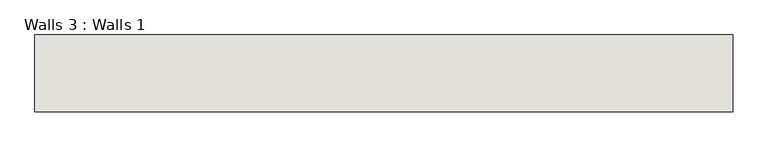
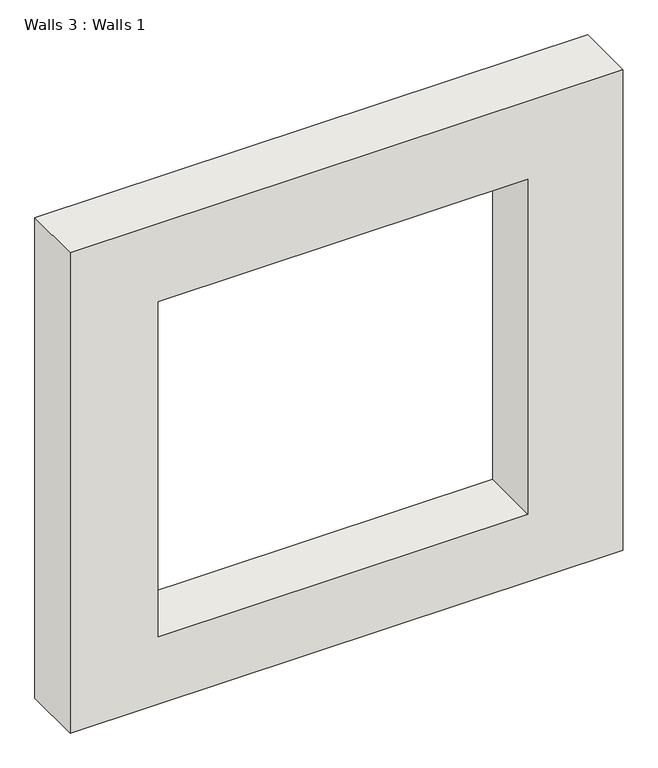
"""IFC4 building model written with IfcOpenShell, lengths in millimetres: wall geometry, Walls 3 : Walls 1."""

from ifc_helpers import new_model, si_unit, frame, origin, place, context, project, spatial, polyline, outline, extrude, source, transform, mapped, element, save


def walls_3_walls_1_8b7cdd2a(model_context):
    return source(origin(), model_context, "Body", "SweptSolid", [
        extrude(outline(polyline([(10639.5789316, -6069.6817469), (10639.5789316, -8558.8817469), (8353.5789316, -8558.8817469), (8353.5789316, -6069.6817469), (10639.5789316, -6069.6817469)]), holes=[polyline([(10268.0681256, -6498.1357575), (8674.2181256, -6498.1357575), (8674.2181256, -8161.8357575), (10268.0681256, -8161.8357575), (10268.0681256, -6498.1357575)])]), frame((0.0, 1408.0209854, 0.0), z_axis=(0.0, 1.0, 0.0), x_axis=(0.0, 0.0, 1.0)), (0.0, 0.0, 1.0), 274.2274628),
    ])


if __name__ == "__main__":
    model = new_model("IFC4")
    model_context = context("Model", 3, world=origin())
    ifc_project = project(units=[si_unit("LENGTHUNIT", "METRE", prefix="MILLI")], contexts=[model_context])
    site = spatial("IfcSite", under=ifc_project)
    building = spatial("IfcBuilding", under=site)
    placement = place(None, origin())
    walls_3_walls_1_shape = walls_3_walls_1_8b7cdd2a(model_context)
    element("IfcWall", 1, ObjectType="Walls 3 : Walls 1", at=placement, inside=building, context=model_context, shape_type="MappedRepresentation", body=[
        mapped(walls_3_walls_1_shape, transform((0.0, 0.0, 0.0), x_axis=(1.0, 0.0, 0.0), y_axis=(0.0, 1.0, 0.0), z_axis=(0.0, 0.0, 1.0))),
    ])
    save(model, "model.ifc")

# Revit data of these elements
# Element 1 (IfcWall, "Walls 3 : Walls 1")
#   Materials on its faces: "Default Wall"
# Materials
#   "Default Wall": colour RGB 128 128 128, transparency 0
